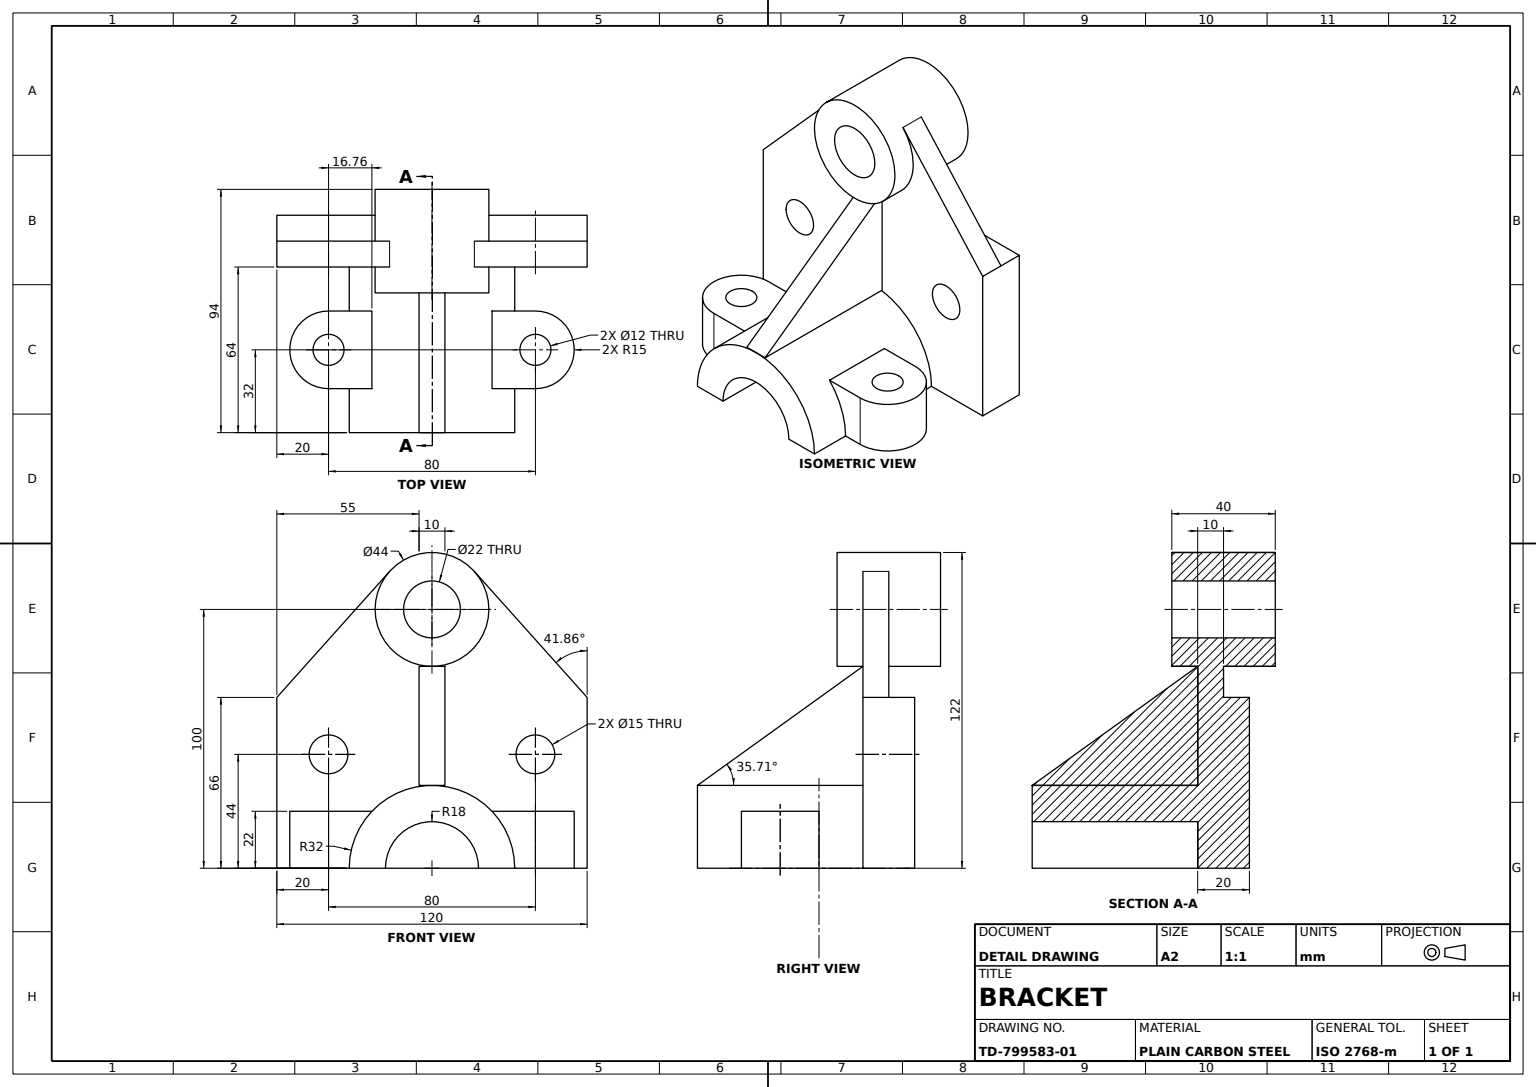
from build123d import *

# Parameters (mm, degrees)
BASE_PLATE_SKETCH_W        = 120
BASE_PLATE_SKETCH_H        = 66
BASE_PLATE_DEPTH           = 20
SADDLE_BOSS_R32_DEPTH      = 64
SADDLE_BORE_R18_DEPTH      = 64
UPRIGHT_PLATE_DEPTH        = 10
EYE_START                  = 10
EYE_BOSS_FRONT_SKETCH_R    = 22
EYE_BOSS_FRONT_44_DEPTH    = 10
EYE_BOSS_REAR_SKETCH_R     = 22
EYE_BOSS_REAR_44_DEPTH     = 20
EYE_BORE_SKETCH_R          = 11
EYE_BORE_22_DEPTH          = 50
SADDLE_MOUNTING_LUGS_DEPTH = 22
PLATE_RELIEF_SKETCH_R      = 7.5
PLATE_RELIEF_CUT_DEPTH     = 30
RIB_BLOCK_DEPTH            = 120
RIB_TRIM_SIDE_A_DEPTH      = 55
RIB_TRIM_SIDE_B_DEPTH      = 55
LUG_HOLES_SKETCH_R         = 6
LUG_HOLES_2X_12_DEPTH      = 55


with BuildPart() as part:
    # Base Plate Sketch → Base Plate (new body)
    with BuildSketch(Plane.XY):
        with Locations((60, 33)):
            Rectangle(BASE_PLATE_SKETCH_W, BASE_PLATE_SKETCH_H)
    extrude(amount=-BASE_PLATE_DEPTH)

    # Saddle Boss Sketch → Saddle Boss R32 (add)
    with BuildSketch(Plane.XY):
        with BuildLine():
            Line((28, 0), (92, 0))
            ThreePointArc((92, 0), (60, 32), (28, 0))
        make_face()
    extrude(amount=SADDLE_BOSS_R32_DEPTH)

    # Saddle Bore Sketch → Saddle Bore R18 (cut)
    with BuildSketch(Plane.XY.offset(64)):
        with BuildLine():
            Line((42, 0), (78, 0))
            ThreePointArc((78, 0), (60, 18), (42, 0))
        make_face()
    extrude(amount=-SADDLE_BORE_R18_DEPTH, mode=Mode.SUBTRACT)

    # Upright Plate Sketch → Upright Plate (add)
    with BuildSketch(Plane.XY):
        with BuildLine():
            Line((0, 66), (120, 66))
            Line((120, 66), (76.38555148, 114.680384964))
            ThreePointArc((76.38555148, 114.680384964), (60, 122), (43.61444852, 114.680384964))
            Line((43.61444852, 114.680384964), (0, 66))
        make_face()
    extrude(amount=-UPRIGHT_PLATE_DEPTH)

    # Eye Boss Front Sketch → Eye Boss Front Ø44 (add)
    with BuildSketch(Plane.XY.offset(EYE_START)):
        with Locations((60, 100)):
            Circle(EYE_BOSS_FRONT_SKETCH_R)
    extrude(amount=-EYE_BOSS_FRONT_44_DEPTH)

    # Eye Boss Rear Sketch → Eye Boss Rear Ø44 (add)
    with BuildSketch(Plane(origin=(0, 0, -10), x_dir=(-1, 0, 0), z_dir=(0, 0, -1))):
        with Locations(Location((-60, 100, 0), (0, 0, 180))):
            Circle(EYE_BOSS_REAR_SKETCH_R)
    extrude(amount=EYE_BOSS_REAR_44_DEPTH)

    # Eye Bore Sketch → Eye Bore Ø22 (cut)
    with BuildSketch(Plane.XY.offset(10)):
        with Locations((60, 100)):
            Circle(EYE_BORE_SKETCH_R)
    extrude(amount=-EYE_BORE_22_DEPTH, mode=Mode.SUBTRACT)

    # Mounting Lugs Sketch → Saddle Mounting Lugs (add)
    with BuildSketch(Plane.XZ):
        with BuildLine():
            Line((20, 47), (42, 47))
            Line((42, 47), (42, 17))
            Line((42, 17), (20, 17))
            ThreePointArc((20, 17), (5, 32), (20, 47))
        make_face()
        with BuildLine():
            Line((100, 47), (78, 47))
            Line((78, 47), (78, 17))
            Line((78, 17), (100, 17))
            ThreePointArc((100, 17), (115, 32), (100, 47))
        make_face()
    extrude(amount=-SADDLE_MOUNTING_LUGS_DEPTH)

    # Plate Relief Sketch → Plate Relief Cut (cut)
    with BuildSketch(Plane.XY):
        with Locations((20, 44)):
            Circle(PLATE_RELIEF_SKETCH_R)
        with Locations((100, 44)):
            Circle(PLATE_RELIEF_SKETCH_R)
    extrude(amount=-PLATE_RELIEF_CUT_DEPTH, mode=Mode.SUBTRACT)

    # Lug Holes Sketch → Lug Holes 2xØ12 (cut)
    with BuildSketch(Plane(origin=(0, 22, 0), x_dir=(1, 0, 0), z_dir=(0, 1, 0))):
        with Locations(Location((20, -32, 0), (0, 0, 270))):
            Circle(LUG_HOLES_SKETCH_R)
        with Locations(Location((100, -32, 0), (0, 0, 270))):
            Circle(LUG_HOLES_SKETCH_R)
    extrude(amount=-LUG_HOLES_2X_12_DEPTH, mode=Mode.SUBTRACT)


with BuildPart() as body_2:
    # Rib Block Sketch → Rib Block (new body)
    with BuildSketch(Plane.ZY):
        Polygon((0, 78), (64, 32), (0, 32), align=None)
    extrude(amount=-RIB_BLOCK_DEPTH)

    # Rib Trim Side A Sketch → Rib Trim Side A (cut)
    with BuildSketch(Plane.ZY):
        Polygon((0, 78), (64, 32), (0, 32), align=None)
    extrude(amount=-RIB_TRIM_SIDE_A_DEPTH, mode=Mode.SUBTRACT)

    # Rib Trim Side B Sketch → Rib Trim Side B (cut)
    with BuildSketch(Plane(origin=(120, 0, 0), x_dir=(0, 0, -1), z_dir=(1, 0, 0))):
        Polygon((0, 78), (-64, 32), (0, 32), align=None)
    extrude(amount=-RIB_TRIM_SIDE_B_DEPTH, mode=Mode.SUBTRACT)


solid = Compound([part.part, body_2.part])
